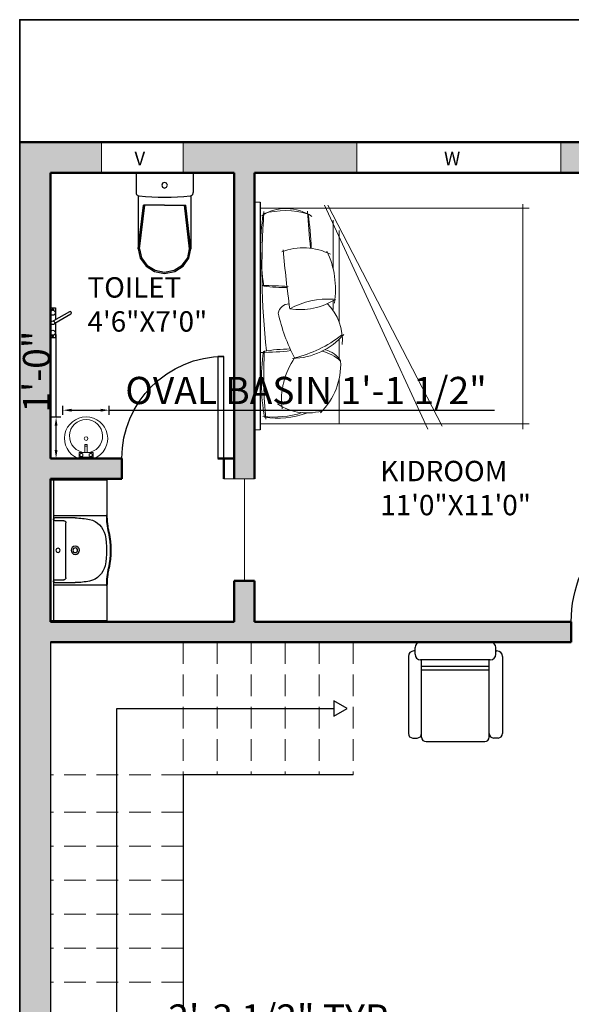
# Model space of a CAD drawing. Units: inches. Extents: x 3354 to 4308, y 1668 to 2317.
# Tile 10 of 11: x 3871 to 4033, y 2005 to 2294. Entities that reach past the tile are written whole.
import ezdxf

# ---------------------------------------------------------------- set-up
doc = ezdxf.new("R2010")
doc.units = ezdxf.units.IN
doc.linetypes.add('DASHED', pattern=[19.05, 12.7, -6.35])
for name, color, linetype, lineweight in [('0.10', 252, 'Continuous', 9), ('A-ANNO-DIMS', 2, 'Continuous', 18), ('A-ANNO-TEXT', 7, 'Continuous', 18), ('A-AREA-IDEN', 3, 'Continuous', 18), ('A-DOOR', 3, 'Continuous', 25), ('A-FLOR-FIXT', 8, 'Continuous', 18), ('A-FLOR-OVHD', 8, 'DASHED', 18), ('A-FLOR-STRS', 7, 'Continuous', 25), ('A-FURN', 8, 'Continuous', 18), ('A-GLAZ', 4, 'Continuous', 18), ('A-WALL', 7, 'Continuous', 50), ('A-WALL-PATT', 8, 'Continuous', 13), ('C-PROP', 1, 'Continuous', 35)]:
    doc.layers.add(name, color=color, linetype=linetype, lineweight=lineweight)
doc.layers.add('SANTEH', color=7, linetype='Continuous')
doc.layers.add('wood', color=26, linetype='Continuous')
doc.styles.get("Standard").update_dxf_attribs({"font": 'arial.ttf'})
doc.dimstyles.new('ISO-25', dxfattribs={"dimtxt": 8, "dimasz": 2.5, "dimexe": 1.25, "dimexo": 0.625, "dimtad": 1, "dimdec": 1, "dimlunit": 3, "dimtxsty": 'Standard', "dimcen": 2.5, "dimadec": 0, "dimazin": 0, "dimtfac": 1, "dimtdec": 1, "dimtmove": 0, "dimatfit": 3, "dimfxl": 1, "dimarcsym": 0})

# ---------------------------------------------------------------- blocks, each defined once
blk = doc.blocks.new('*U2')
for p, q in [((0, 0), (0, -6)), ((30, 0), (30, -6))]:
    blk.add_line(p, q)
blk.add_lwpolyline([(0, 0), (0, 30), (1.75, 30), (1.75, 0)], close=True)
blk.add_arc((0, 0), 30, 0, 90)
blk = doc.blocks.new('WC 2 Symb_109')
at = {"layer": 'SANTEH'}
for p, q in [((0, 0), (0, 380)), ((0, 380), (132.4, 380)), ((153.6, 364.9), (506.8, 364.9)), ((506.3, 364.9), (215.7, 330.9)), ((506.3, 356), (215.7, 322)), ((215.7, 190), (215.7, 330.9)), ((215.7, 190), (215.7, 49.1)), ((153.8, 15.1), (506.8, 15.1)), ((506.3, 24), (215.7, 58)), ((506.3, 15.1), (215.7, 49.1)), ((0, 0), (132.4, 0))]:
    blk.add_line(p, q, dxfattribs=at)
for points in [[(154.6, 360.1), (153.9, 364.1), (152.3, 367.9), (150.2, 371.3), (147.4, 374.3), (144.1, 376.7), (140.5, 378.5), (136.5, 379.6), (132.4, 380)], [(154.6, 19.7), (158.6, 62.1), (161.4, 104.7), (163.1, 147.3), (163.7, 189.9), (163.1, 232.5), (161.4, 275.1), (158.6, 317.7), (154.6, 360.1)], [(506.3, 24), (565.5, 36.6), (615.7, 72.6), (649.2, 126.5), (661, 190), (649.2, 253.5), (615.7, 307.4), (565.5, 343.4), (506.3, 356)], [(506.8, 15.1), (569.2, 28.4), (622.2, 66.3), (657.6, 123.1), (670, 190), (657.6, 256.9), (622.2, 313.7), (569.2, 351.6), (506.8, 364.9)], [(132.4, 0), (136.5, 0.4), (140.4, 1.5), (144.1, 3.2), (147.3, 5.6), (150.1, 8.6), (152.3, 12), (153.8, 15.7), (154.6, 19.7)]]:
    blk.add_lwpolyline(points, dxfattribs=at)
blk.add_lwpolyline([(83.6, 208.5), (70.4, 203.1), (64.9, 190), (70.4, 176.9), (83.6, 171.5), (96.8, 176.9), (102.2, 190), (96.8, 203.1)], close=True, dxfattribs=at)
blk = doc.blocks.new('Faucet - kit sink top')
at = {"layer": 'SANTEH'}
for p, q in [((-5.5, -0.75), (-5.5, -1.25)), ((-4.94278, -0.75), (-5.5, -0.75)), ((-5.5, -1.25), (-4.94278, -1.25)), ((-0.14775, -1.7441), (3.56698, -8.1782)), ((4.43301, -7.6782), (0.71828, -1.2441)), ((4.94278, -0.75), (5.5, -0.75)), ((5.5, -1.25), (4.94278, -1.25)), ((5.5, -0.75), (5.5, -1.25))]:
    blk.add_line(p, q, dxfattribs=at)
blk.add_lwpolyline([(-0.00587, -2), (-6, -2), (-6, 0), (6, 0), (6, -2), (1.15195, -2)], dxfattribs=at)
for centre, radius in [((-4, -1), 1), ((4, -1), 1), ((0, -1), 0.75)]:
    blk.add_circle(centre, radius, dxfattribs=at)
blk.add_arc((4, -7.9282), 0.5, 210, 30, dxfattribs=at)
blk = doc.blocks.new('s_02')
at = {"layer": 'SANTEH'}
for p, q in [((0, 0), (-519.4, -1.7)), ((0, 0), (-519.4, -1.7)), ((-520.5, -2.8), (-519.8, -209.5)), ((-520.5, -2.8), (-519.8, -209.5)), ((-517.6, -207.3), (-518.3, -5)), ((-1, -11.7), (-518.3, -13.5)), ((-517.2, -3.9), (-2.2, -2.2)), ((-387.2, -207.9), (-387.9, -13)), ((-378.3, -17.4), (-378.1, -92.6)), ((-368.3, -17.3), (-368.2, -50.3)), ((-150.9, -49.6), (-151, -16.6)), ((-140.7, -91.8), (-141, -16.6)), ((-131.4, -12.2), (-130.8, -207.1)), ((-1.1, -3.3), (-0.4, -205.6)), ((1.8, -207.7), (1.1, -1.1)), ((1.8, -207.7), (1.1, -1.1)), ((-360.4, -58.1), (-158.7, -57.4)), ((-518.7, -210.5), (-389.4, -210.1)), ((-518.7, -210.5), (-389.4, -210.1)), ((-389.4, -207.9), (-516.6, -208.4)), ((-1.5, -206.6), (-128.6, -207.1)), ((-128.6, -209.2), (0.7, -208.8)), ((-128.6, -209.2), (0.7, -208.8))]:
    blk.add_line(p, q, dxfattribs=at)
at = {"layer": 'SANTEH', "extrusion": (0, 0, -1)}
for centre, major_axis, ratio, start_param, end_param in [((0, -1.1), (-0.38, 1.02), 0.991976, 0.357514, 1.923061), ((0, -1.1), (-0.38, 1.02), 0.991976, 0.357514, 1.923061), ((-519.4, -2.8), (0, -1.09), 0.99914, 1.570796, 3.141593), ((-519.4, -2.8), (0, -1.09), 0.99914, 1.570796, 3.141593), ((-517.2, -5), (0, -1.09), 0.99914, 1.570796, 3.141593), ((-374, -17.3), (0.01, -4.35), 0.99914, 1.570796, 3.141593), ((-372.7, -17.3), (0.01, -4.35), 0.99914, 3.141593, 4.712389), ((-259.6, -29.1), (0.03, -7.61), 0.99914, 1.570796326742688, 7.853981633922275), ((-146.6, -16.6), (0.01, -4.35), 0.99914, 1.570796, 3.141593), ((-145.3, -16.6), (0.01, -4.35), 0.99914, 3.141593, 4.712389), ((-2.2, -3.3), (0, -1.09), 0.99914, 3.141593, 4.712389), ((-360.4, -50.3), (0.03, -7.83), 0.99914, 0, 1.570796), ((-158.7, -49.6), (0.03, -7.83), 0.99914, -1.570796, 0), ((-128, -91.8), (0.8, -250.2), 0.99914, 1.359365, 1.570796), ((-259.4, -92.2), (0.1, -15.2), 0.99914, 1.570796326791235, 7.853981633970821), ((-259.4, -92.2), (0.03, -8.7), 0.99914, 1.570796326873691, 7.853981634053277), ((-390.8, -92.7), (0.8, -250.2), 0.99914, -1.570796, -1.359365), ((-218.1, -129.1), (0.2, -73.7), 0.99914, -1.359365, -0.211723), ((-300.4, -129.4), (0.2, -73.7), 0.99914, 0.211723, 1.359365), ((-518.7, -209.5), (0, -1.09), 0.99914, 0, 1.570796), ((-518.7, -209.5), (0, -1.09), 0.99914, 0, 1.570796), ((-516.6, -207.3), (0, -1.09), 0.99914, 0, 1.570796), ((-388.3, -539.7), (1.1, -331.7), 0.99914, 3.141593, 3.34093), ((-388.3, -539.7), (1.1, -329.5), 0.99914, 3.141593, 3.34093), ((-388.3, -539.7), (1.1, -329.5), 0.99914, 3.141593, 3.34093), ((-260.1, 106.8), (1.1, -329.5), 0.99914, -0.199337, 0.199337), ((-260.1, 106.8), (1.1, -329.5), 0.99914, -0.199337, 0.199337), ((-260.1, 106.8), (1.1, -327.4), 0.99914, -0.199337, 0.199337), ((-259.9, 62.3), (0.9, -269.6), 0.99914, -0.211723, 0.211723), ((-127.5, -538.8), (1.1, -331.7), 0.99914, 2.942255, 3.141593), ((-127.5, -538.8), (1.1, -329.5), 0.99914, 2.942255, 3.141593), ((-127.5, -538.8), (1.1, -329.5), 0.99914, 2.942255, 3.141593), ((-1.5, -205.6), (0, -1.09), 0.99914, 4.712389, 6.283185), ((0.7, -207.7), (0, -1.09), 0.99914, 4.712389, 6.283185), ((0.7, -207.7), (0, -1.09), 0.99914, 4.712389, 6.283185)]:
    blk.add_ellipse(centre, major_axis=major_axis, ratio=ratio, start_param=start_param, end_param=end_param, dxfattribs=at)
blk = doc.blocks.new('A$C38B70996')
at = {"layer": 'wood'}
for p, q in [((0.11, 0.9), (0.74, 0.9)), ((0.06, 0.82), (0.05, 0.82)), ((0.06, 0.79), (0.06, 0.85)), ((0.79, 0.79), (0.79, 0.85)), ((0.79, 0.82), (0.8, 0.82)), ((0, 0.77), (0, 0.073)), ((0.74, 0.74), (0.11, 0.74)), ((0.12, 0.04), (0.12, 0.74)), ((0.73, 0.04), (0.73, 0.74)), ((0.85, 0.77), (0.85, 0.073)), ((0.73, 0.68), (0.12, 0.68)), ((0.73, 0.647), (0.12, 0.647)), ((0.04, 0.033), (0.08, 0.033)), ((0.16, 0), (0.69, 0)), ((0.81, 0.033), (0.77, 0.033))]:
    blk.add_line(p, q, dxfattribs=at)
for centre, radius, start, end in [((0.11, 0.85), 0.05, 90, 180), ((0.74, 0.85), 0.05, 0, 90), ((0.05, 0.77), 0.05, 90, 180), ((0.8, 0.77), 0.05, 360, 90), ((0.11, 0.79), 0.05, 180, 270), ((0.74, 0.79), 0.05, 270, 0), ((0.04, 0.073), 0.04, 180, 270), ((0.08, 0.073), 0.04, 270, 0), ((0.16, 0.04), 0.04, 180, 270), ((0.69, 0.04), 0.04, 270, 360), ((0.77, 0.073), 0.04, 180, 270), ((0.81, 0.073), 0.04, 270, 360)]:
    blk.add_arc(centre, radius, start, end, dxfattribs=at)
blk = doc.blocks.new('*U3')
for p, q in [((0, 0), (0, -6)), ((36, 0), (36, -6))]:
    blk.add_line(p, q)
blk.add_lwpolyline([(0, 0), (0, 36), (1.75, 36), (1.75, 0)], close=True)
blk.add_arc((0, 0), 36, 0, 90)
blk = doc.blocks.new('M_BATH_BASIN_Basin - Oval_P')
at = {"color": 0, "linetype": 'ByBlock', "lineweight": -2}
blk.add_lwpolyline([(0, 90, -5.027337), (0, -90)], format="xyb", close=True, dxfattribs=at)
blk.add_lwpolyline([(63, 12, -30), (63, -12, -1.097889)], format="xyb", dxfattribs=at)
for points in [[(13, -76), (13, 76), (63, 76), (63, -76)], [(19, 51), (29, 67), (48, 67), (57, 51), (48, 34), (29, 34)]]:
    blk.add_lwpolyline(points, close=True, dxfattribs=at)
for points in [[(63, 12), (152, 12), (152, -12), (63, -12)], [(134, 12), (134, -12)], [(29, -34), (48, -34), (57, -51), (48, -67), (29, -67), (19, -51), (29, -34)]]:
    blk.add_lwpolyline(points, dxfattribs=at)
blk.add_circle((216, 0), 20.1, dxfattribs=at)
at = {"layer": 'Defpoints'}
for p in [(0, 234), (0, -234)]:
    blk.add_point(p, dxfattribs=at)
blk = doc.blocks.new('camita')
at = {"layer": '0.10'}
for p, q in [((-0.85, -0.045), (0.85, -0.045)), ((-0.805, -0.045), (-0.805, -2.0485)), ((0.805, -0.045), (0.805, -2.0485)), ((-0.8271, -0.521), (0.8464, -1.2932)), ((-0.8271, -0.5476), (0.8236, -1.3992)), ((-0.7161, -0.585), (-0.3554, -0.585)), ((-0.1136, -0.585), (-0.0485, -0.585)), ((-0.638, -0.63), (0.0434, -0.63)), ((0.1749, -0.63), (0.3179, -0.63)), ((0.4739, -0.63), (0.805, -0.63)), ((-0.8354, -2), (0.8464, -2))]:
    blk.add_line(p, q, dxfattribs=at)
blk.add_lwpolyline([(-0.85, -0.0405), (0.85, -0.0405), (0.85, 0), (-0.85, 0)], close=True, dxfattribs=at)
for centre, radius, start, end in [((-0.4574, -0.2364), 0.3443, 147.50996, 213.83359), ((-0.1997, -0.2266), 0.5864, 163.92635, 197.14087), ((-0.3639, -5.8457), 5.7909, 83.80731, 94.12107), ((-0.5104, -1.7232), 1.6781, 80.12554, 98.66187), ((2.3534, -0.0532), 2.5803, 180.10628, 184.38541), ((-1.5443, -0.2452), 1.3333, 359.93941, 7.55329), ((1.5815, -0.2893), 1.3353, 170.38021, 178.99138), ((-1.4396, -0.0609), 1.7117, 352.92911, 0.39592), ((0.4524, -3.0675), 2.9996, 83.90257, 93.67595), ((0.4863, -1.6286), 1.5781, 80.16015, 98.05996), ((0.0294, -0.1377), 0.7262, 342.58415, 6.00484), ((0.1326, -0.1696), 0.6307, 339.92303, 8.74334), ((-0.0543, -0.3633), 0.4542, 159.30257, 206.50263), ((-1.3301, -9.6748), 9.4985, 82.27078, 84.93989), ((-0.007, -0.258), 0.0828, 100.01798, 179.73597), ((-0.2931, -1.4378), 1.2903, 61.97485, 77.84351), ((0.6265, -0.7518), 0.5508, 82.96906, 124.67388), ((0.3203, -0.3944), 0.4043, 341.45245, 33.45121), ((0.4585, -0.5454), 0.5842, 151.04555, 184.14969), ((-0.5341, -0.3393), 0.4875, 327.26442, 9.0473), ((-0.1986, -0.2742), 0.5159, 310.73945, 359.05759), ((-0.5673, -0.0868), 0.9057, 321.69527, 346.46261), ((-1.8672, -14.986), 14.6323, 84.65974, 85.75157), ((-0.4598, 1.4861), 1.9092, 260.95299, 268.65169), ((0.5707, -0.4317), 0.3145, 192.93877, 221.96363), ((0.3612, -0.133), 0.5096, 267.25889, 315.29965), ((-0.2002, 0.064), 0.6673, 244.78094, 279.06058), ((0.179, -0.272), 0.3828, 224.52836, 275.22287), ((0.4384, -0.4834), 0.1898, 193.68485, 236.70352)]:
    blk.add_arc(centre, radius, start, end, dxfattribs=at)
blk = doc.blocks.new('*D55')
at = {"layer": 'A-ANNO-DIMS', "color": 0, "lineweight": -2, "transparency": 16777216}
for p, q in [((3985.74, 1994.97), (3914.45, 1994.97)), ((3985.74, 1991.2), (3985.74, 1996.22)), ((4010.89, 1994.97), (3988.24, 1994.97)), ((4013.39, 1991.2), (4013.39, 1996.22))]:
    blk.add_line(p, q, dxfattribs=at)
at = {"layer": 'A-ANNO-DIMS', "color": 0, "transparency": 16777216}
for points in [[(3988.24, 1995.38), (3988.24, 1994.55), (3985.74, 1994.97)], [(4010.89, 1995.38), (4010.89, 1994.55), (4013.39, 1994.97)]]:
    blk.add_solid(points, dxfattribs=at)
at = {"layer": 'Defpoints', "color": 0, "transparency": 16777216}
for p in [(3985.74, 1994.97), (3985.74, 1990.57), (4013.39, 1990.57)]:
    blk.add_point(p, dxfattribs=at)
at = {"layer": 'A-ANNO-DIMS', "color": 0, "transparency": 16777216, "insert": (3948.84, 1999.73), "char_height": 8, "attachment_point": 5}
blk.add_mtext('2\'-3 1/2" TYP.', dxfattribs=at)
blk = doc.blocks.new('*D92')
at = {"layer": 'A-ANNO-DIMS', "color": 0, "lineweight": -2, "transparency": 16777216}
for p, q in [((3884.05, 2178.07), (3884.05, 2180.73)), ((3897.61, 2178.07), (3897.61, 2180.73)), ((3886.55, 2179.48), (3895.11, 2179.48)), ((3897.61, 2179.48), (4010.76, 2179.48))]:
    blk.add_line(p, q, dxfattribs=at)
at = {"layer": 'A-ANNO-DIMS', "color": 0, "transparency": 16777216}
for points in [[(3886.55, 2179.89), (3886.55, 2179.06), (3884.05, 2179.48)], [(3895.11, 2179.89), (3895.11, 2179.06), (3897.61, 2179.48)]]:
    blk.add_solid(points, dxfattribs=at)
at = {"layer": 'Defpoints', "color": 0, "transparency": 16777216}
for p in [(3884.05, 2177.44), (3897.61, 2179.48), (3897.61, 2177.44)]:
    blk.add_point(p, dxfattribs=at)
at = {"layer": 'A-ANNO-DIMS', "color": 0, "transparency": 16777216, "insert": (3955.44, 2184.24), "char_height": 8, "attachment_point": 5}
blk.add_mtext('OVAL BASIN 1\'-1 1/2"', dxfattribs=at)
blk = doc.blocks.new('*D93')
at = {"layer": 'A-ANNO-DIMS', "color": 0, "lineweight": -2, "transparency": 16777216}
for p, q in [((3882.02, 2177.44), (3882.02, 2201.71)), ((3883.43, 2177.44), (3880.77, 2177.44)), ((3882.02, 2167.8), (3882.02, 2174.94)), ((3883.43, 2165.3), (3880.77, 2165.3))]:
    blk.add_line(p, q, dxfattribs=at)
at = {"layer": 'A-ANNO-DIMS', "color": 0, "transparency": 16777216}
for points in [[(3881.6, 2174.94), (3882.44, 2174.94), (3882.02, 2177.44)], [(3881.6, 2167.8), (3882.44, 2167.8), (3882.02, 2165.3)]]:
    blk.add_solid(points, dxfattribs=at)
at = {"layer": 'Defpoints', "color": 0, "transparency": 16777216}
for p in [(3882.02, 2177.44), (3884.05, 2177.44), (3884.05, 2165.3)]:
    blk.add_point(p, dxfattribs=at)
at = {"layer": 'A-ANNO-DIMS', "color": 0, "transparency": 16777216, "insert": (3877.31, 2190.82), "char_height": 8, "attachment_point": 5, "rotation": 90}
blk.add_mtext('1\'-0"', dxfattribs=at)

msp = doc.modelspace()

# ---------------------------------------------------------------- hatches: boundary and pattern name
at = {"layer": 'A-WALL-PATT', "transparency": 33554687}
h = msp.add_hatch(color=256, dxfattribs=at)
h.dxf.hatch_style = 1
h.paths.add_polyline_path([(4078.33, 1991.3), (4069.33, 1991.3), (4069.33, 1961.3), (4063.33, 1961.3), (4063.33, 1955.3), (4069.33, 1955.3), (4069.33, 1808.3), (4078.33, 1808.3), (4078.33, 1829.3), (4108.33, 1829.3), (4108.33, 1838.3), (4078.33, 1838.3)])
h.paths.add_polyline_path([(4219.33, 1850.3), (4210.33, 1850.3), (4210.33, 1838.3), (4180.33, 1838.3), (4180.33, 1829.3), (4219.33, 1829.3)])
h.paths.add_polyline_path([(4219.33, 2075.3), (4210.33, 2075.3), (4210.33, 2039.3), (4206.56, 2039.3), (4138.33, 2039.3), (4138.33, 2042.3), (4132.33, 2042.3), (4132.33, 2009.3), (4138.33, 2009.3), (4138.33, 2033.3), (4210.33, 2033.3), (4210.33, 1985.4), (4211.13, 1985.4), (4211.13, 1969.85), (4211.13, 1902.33), (4211.13, 1898.3), (4219.33, 1898.3)])
h.paths.add_polyline_path([(4078.33, 2111.3), (4132.33, 2111.3), (4132.33, 2072.3), (4138.33, 2072.3), (4138.33, 2111.3), (4210.33, 2111.3), (4210.33, 2099.3), (4219.33, 2099.3), (4219.33, 2150.3), (4210.33, 2150.3), (4210.33, 2117.3), (4078.33, 2117.3), (4078.33, 2249.3), (4108.33, 2249.3), (4108.33, 2258.3), (4030.33, 2258.3), (4030.33, 2249.3), (4072.33, 2249.3), (4072.33, 2117.3), (4069.33, 2117.3), (4069.33, 2111.3), (4069.33, 2027.3), (4075.33, 2027.3), (4078.33, 2027.3), (4078.33, 2033.3), (4102.33, 2033.3), (4102.33, 2039.3), (4078.33, 2039.3)])
h.paths.add_polyline_path([(4219.33, 2258.3), (4180.33, 2258.3), (4180.33, 2249.3), (4210.33, 2249.3), (4210.33, 2210.3), (4219.33, 2210.3)], flags=17)
h.paths.add_polyline_path([(3970.33, 2258.3), (3919.33, 2258.3), (3919.33, 2249.3), (3922.3, 2249.3), (3934.33, 2249.3), (3934.33, 2159.3), (3940.33, 2159.3), (3940.33, 2249.3), (3970.33, 2249.3)], flags=17)
h.paths.add_polyline_path([(3880.33, 2111.3), (4033.33, 2111.3), (4033.33, 2117.3), (3940.33, 2117.3), (3940.33, 2129.3), (3934.33, 2129.3), (3934.33, 2117.3), (3880.33, 2117.3), (3880.33, 2159.3), (3901.33, 2159.3), (3901.33, 2165.3), (3880.33, 2165.3), (3880.33, 2249.3), (3895.33, 2249.3), (3895.33, 2258.3), (3871.33, 2258.3), (3871.33, 1754.3), (3893.83, 1754.3), (3893.83, 1763.3), (3880.33, 1763.3), (3880.33, 1865.3), (3898.33, 1865.3), (3898.33, 1871.3), (3880.33, 1871.3), (3880.33, 1955.3), (3931.33, 1955.3), (3931.33, 1928.3), (3937.33, 1928.3), (3937.33, 1955.3), (4027.33, 1955.3), (4027.33, 1961.3), (3880.33, 1961.3)])
h.paths.add_polyline_path([(3967.33, 1763.3), (3937.33, 1763.3), (3937.33, 1898.3), (3931.33, 1898.3), (3931.33, 1871.3), (3928.33, 1871.3), (3928.33, 1865.3), (3931.33, 1865.3), (3931.33, 1763.3), (3917.83, 1763.3), (3917.83, 1754.3), (3967.33, 1754.3)], flags=17)
h.paths.add_polyline_path([(4078.33, 1772.3), (4069.33, 1772.3), (4069.33, 1763.3), (4039.33, 1763.3), (4039.33, 1754.3), (4078.33, 1754.3)])

# ---------------------------------------------------------------- linework, layer by layer
at = {"layer": 'A-FLOR-OVHD', "ltscale": 0.5}
for p, q in [((3919.33, 2111.3), (3919.33, 2072.3)), ((3929.33, 2111.3), (3929.33, 2072.3)), ((3939.33, 2111.3), (3939.33, 2072.3)), ((3949.33, 2111.3), (3949.33, 2072.3)), ((3959.33, 2111.3), (3959.33, 2072.3)), ((3969.33, 2111.3), (3969.33, 2072.3)), ((3919.33, 2072.3), (3880.33, 2072.3)), ((3919.33, 2061.3), (3880.33, 2061.3)), ((3919.33, 2051.3), (3880.33, 2051.3)), ((3919.33, 2041.3), (3880.33, 2041.3)), ((3919.33, 2031.3), (3880.33, 2031.3)), ((3919.33, 2021.3), (3880.33, 2021.3)), ((3919.33, 2011.3), (3880.33, 2011.3))]:
    msp.add_line(p, q, dxfattribs=at)
at = {"layer": 'A-FLOR-STRS'}
for p, q in [((3880.33, 2111.3), (3880.33, 1961.3)), ((3969.33, 2072.3), (3919.33, 2072.3)), ((3919.33, 2072.3), (3919.33, 1961.3))]:
    msp.add_line(p, q, dxfattribs=at)
msp.add_lwpolyline([(3967.49, 2091.8), (3963.6, 2094.04), (3963.6, 2089.55)], close=True, dxfattribs=at)
msp.add_lwpolyline([(3969.33, 1980.8), (3899.83, 1980.8), (3899.83, 2091.8), (3963.6, 2091.8)], dxfattribs=at)
at = {"layer": 'A-FURN'}
msp.add_line((3937.33, 2129.3), (3937.33, 2159.3), dxfattribs=at)
at = {"layer": 'A-GLAZ'}
for p, q in [((3895.33, 2249.3), (3895.33, 2258.3)), ((3919.33, 2249.3), (3919.33, 2258.3)), ((3970.33, 2249.3), (3970.33, 2258.3)), ((4030.33, 2249.3), (4030.33, 2258.3)), ((3940.33, 2159.3), (3931.33, 2159.3))]:
    msp.add_line(p, q, dxfattribs=at)
at = {"layer": 'A-WALL'}
for p, q in [((4219.33, 2258.3), (3871.33, 2258.3)), ((3880.33, 2249.3), (3880.33, 2165.3)), ((3934.33, 2249.3), (3880.33, 2249.3)), ((3934.33, 2159.3), (3934.33, 2249.3)), ((4072.33, 2249.3), (3940.33, 2249.3)), ((3940.33, 2159.3), (3940.33, 2249.3)), ((3901.33, 2165.3), (3880.33, 2165.3)), ((3901.33, 2159.3), (3901.33, 2165.3)), ((3934.33, 2165.3), (3929.58, 2165.3)), ((3931.33, 2159.3), (3931.33, 2165.3)), ((3934.33, 2165.3), (3931.33, 2165.3)), ((3901.33, 2159.3), (3880.33, 2159.3)), ((3880.33, 2159.3), (3880.33, 2117.3)), ((3934.33, 2117.3), (3934.33, 2129.3)), ((3940.33, 2129.3), (3934.33, 2129.3)), ((3940.33, 2117.3), (3940.33, 2129.3)), ((3934.33, 2117.3), (3880.33, 2117.3)), ((4033.33, 2117.3), (3940.33, 2117.3)), ((4033.33, 2111.3), (4033.33, 2117.3)), ((4033.33, 2111.3), (3880.33, 2111.3))]:
    msp.add_line(p, q, dxfattribs=at)
at = {"layer": 'C-PROP'}
msp.add_lwpolyline([(4255.33, 1754.3), (4255.33, 2294.3), (3871.33, 2294.3), (3871.33, 1754.3), (4255.33, 1754.3)], dxfattribs=at)

# ---------------------------------------------------------------- block references
at = {"layer": 'A-DOOR', "xscale": -1}
for name, p in [('*U2', (3931.33, 2165.3)), ('*U3', (4069.33, 2117.3))]:
    msp.add_blockref(name, p, dxfattribs=at)
at = {"layer": 'A-FLOR-FIXT'}
for name, p, xscale, yscale, zscale, rotation in [('WC 2 Symb_109', (3905.51, 2249.3), 0.0441898926459964, 0.0441898926459964, 0.0441898926459964, 269.9999999999999), ('Faucet - kit sink top', (3880.33, 2205.18), 0.7356136897818673, 0.7356136897818673, 0.7356136897818673, 90), ('M_BATH_BASIN_Basin - Oval_P', (3890.83, 2165.3), -0.0269806523403052, 0.0269806523403052, 0.0269806523403052, 270), ('s_02', (3880.34, 2159.09), 0.0800758531328607, 0.0800758531328607, 0.0800758531328607, 89.80836855164229)]:
    msp.add_blockref(name, p, dxfattribs=dict(at, xscale=xscale, yscale=yscale, zscale=zscale, rotation=rotation))
at = {"layer": 'A-FURN', "xscale": -39.375, "yscale": 39.375, "zscale": 39.375, "rotation": 90}
msp.add_blockref('camita', (3940.33, 2207.2), dxfattribs=at)
at = {"layer": 'A-FURN', "xscale": 32.53084308163255, "yscale": 32.53084308163255, "zscale": 32.53084308163255}
msp.add_blockref('A$C38B70996', (3985.5, 2082.02), dxfattribs=at)

# ---------------------------------------------------------------- texts
at = {"layer": 'A-ANNO-TEXT', "char_height": 4, "attachment_point": 1}
for s, insert in [('\\pxt6;{V}', (3905.04, 2255.52)), ('\\pxt6;{W}', (3995.97, 2255.52))]:
    msp.add_mtext_dynamic_manual_height_columns(s, width=32.7844, gutter_width=12.5, heights=[0], dxfattribs=dict(at, insert=insert))
at = {"layer": 'A-AREA-IDEN', "char_height": 6, "attachment_point": 1}
for s, insert in [('TOILET\\P4\'6"X7\'0"', (3891.25, 2218.58)), ('KIDROOM\\P11\'0"X11\'0"', (3977.26, 2164.59))]:
    msp.add_mtext_dynamic_manual_height_columns(s, width=74.5832, gutter_width=12.5, heights=[0], dxfattribs=dict(at, insert=insert))

# ---------------------------------------------------------------- dimensions: what is measured, and where the dimension line sits
at = {"layer": 'A-ANNO-DIMS'}
dim = msp.add_linear_dim(base=(3897.61, 2179.48), p1=(3884.05, 2177.44), p2=(3897.61, 2177.44), text='OVAL BASIN <>', dimstyle='ISO-25', override={"dimdec": 1, "dimrnd": 0, "dimzin": 1, "dimlunit": 4, "dimfrac": 2}, dxfattribs=at)
dim.commit()
dim.dimension.update_dxf_attribs({"geometry": '*D92', "text_midpoint": (3955.44, 2184.24)})
dim = msp.add_linear_dim(base=(3882.02, 2177.44), p1=(3884.05, 2165.3), p2=(3884.05, 2177.44), angle=90, dimstyle='ISO-25', override={"dimdec": 1, "dimrnd": 0, "dimzin": 1, "dimlunit": 4, "dimfrac": 2}, dxfattribs=at)
dim.commit()
dim.dimension.update_dxf_attribs({"geometry": '*D93', "text_midpoint": (3877.31, 2190.82)})
dim = msp.add_linear_dim(base=(3985.7374, 1994.9659), p1=(4013.3886, 1990.5742), p2=(3985.7374, 1990.5742), angle=180, text='<> TYP.', dimstyle='ISO-25', override={"dimdec": 1, "dimrnd": 0, "dimzin": 1, "dimlunit": 4, "dimfrac": 2}, dxfattribs=at)
dim.commit()
dim.dimension.update_dxf_attribs({"geometry": '*D55', "text_midpoint": (3948.8416, 1999.7301)})

doc.saveas('drawing.dxf')
